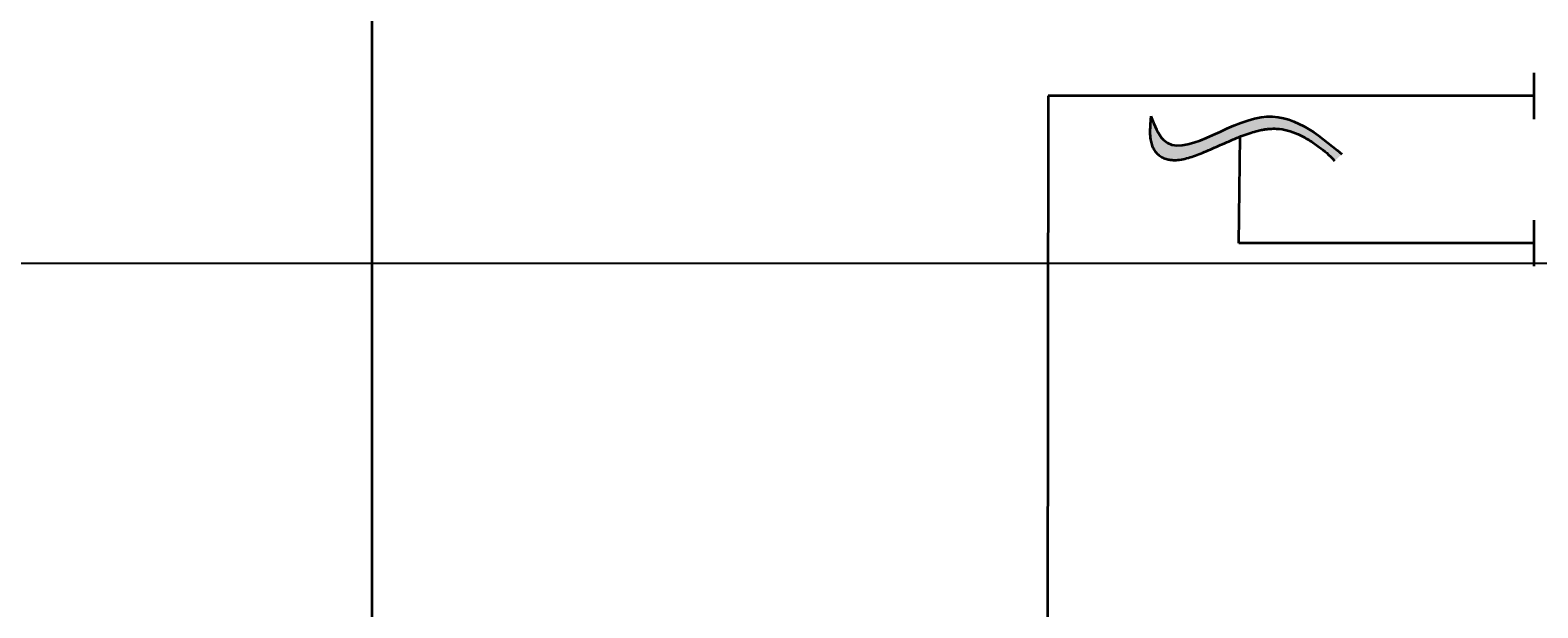
# Model space of a CAD drawing. Units: millimetres. Extents: x 353872 to 441597, y 126154 to 187356.
# Tile 16 of 28: x 391248 to 399262, y 158230 to 161299. Entities that reach past the tile are written whole.
import ezdxf

# ---------------------------------------------------------------- set-up
doc = ezdxf.new("R2010")
doc.units = ezdxf.units.MM
for name, color, linetype, lineweight in [('A-ANNO-DIMS', 2, 'Continuous', 18), ('P-PIPE', 3, 'Continuous', 35), ('P-SYMB-PATT', 8, 'Continuous', 13)]:
    doc.layers.add(name, color=color, linetype=linetype, lineweight=lineweight)
doc.styles.get("Standard").update_dxf_attribs({"font": 'arial.ttf'})
doc.dimstyles.get("Standard").update_dxf_attribs({"dimtxt": 0.18, "dimasz": 0.18, "dimexe": 0.18, "dimexo": 0.0625, "dimgap": 0.09, "dimtad": 0, "dimtih": 1, "dimtoh": 1, "dimdec": 4, "dimzin": 0, "dimdsep": 46, "dimtxsty": 'Standard', "dimcen": 0.09, "dimadec": 0, "dimazin": 0, "dimtfac": 1, "dimtdec": 4, "dimtofl": 0, "dimtmove": 0, "dimatfit": 3, "dimfxl": 1, "dimtolj": 1, "dimtzin": 0, "dimarcsym": 0})

# ---------------------------------------------------------------- blocks, each defined once
blk = doc.blocks.new('*D34')
at = {"layer": 'A-ANNO-DIMS', "color": 0, "lineweight": -2, "transparency": 16777216}
for p, q in [((399457.1, 167930), (356736.4, 167930)), ((356736.5, 167929.8), (356736.5, 163994.3)), ((356736.5, 160058.4), (356736.5, 163993.9)), ((399457.1, 160058.2), (356736.4, 160058.2))]:
    blk.add_line(p, q, dxfattribs=at)
at = {"layer": 'A-ANNO-DIMS', "color": 0, "transparency": 16777216}
for points in [[(356736.5, 167929.8), (356736.6, 167929.8), (356736.5, 167930)], [(356736.5, 160058.4), (356736.6, 160058.4), (356736.5, 160058.2)]]:
    blk.add_solid(points, dxfattribs=at)
at = {"layer": 'Defpoints', "color": 0, "transparency": 16777216}
for p in [(399457.2, 167930), (356736.5, 160058.2), (399457.2, 160058.2)]:
    blk.add_point(p, dxfattribs=at)
at = {"layer": 'A-ANNO-DIMS', "color": 0, "transparency": 16777216, "insert": (356736.5, 163994.1), "char_height": 0.18, "attachment_point": 5}
blk.add_mtext('\\A1;7872', dxfattribs=at)

msp = doc.modelspace()

# ---------------------------------------------------------------- hatches: boundary and pattern name
at = {"layer": 'P-SYMB-PATT'}
h = msp.add_hatch(color=256, dxfattribs=at)
h.dxf.hatch_style = 1
edge = h.paths.add_edge_path()
edge.add_spline(control_points=[(397205.05, 160842.23), (397204.61, 160837.28), (397204.16, 160832.26), (397202.84, 160817.1), (397202.01, 160806.84), (397200.63, 160785.35), (397200.12, 160774.12), (397199.95, 160751.62), (397200.28, 160740.37), (397202.07, 160722.7), (397202.95, 160716.44), (397205.13, 160705.42), (397206.25, 160700.71), (397209.06, 160691.15), (397210.73, 160686.4), (397215.91, 160673.98), (397219.95, 160666.4), (397229.78, 160652.11), (397235.58, 160645.42), (397248.52, 160633.66), (397255.64, 160628.59), (397270.38, 160620.36), (397277.98, 160617.19), (397293.04, 160612.45), (397300.51, 160610.88), (397315.1, 160608.89), (397322.23, 160608.47), (397342.23, 160608.42), (397354.76, 160609.77), (397379.55, 160614.04), (397391.81, 160616.99), (397416.54, 160624.05), (397428.98, 160628.15), (397454.23, 160637.22), (397467.03, 160642.19), (397507.59, 160658.66), (397536.01, 160671.23), (397593.65, 160696.76), (397622.85, 160709.71), (397680.46, 160733.58), (397708.87, 160744.49), (397748.65, 160757.34), (397761.14, 160760.99), (397781.84, 160766.23), (397790.28, 160768.11), (397805.08, 160770.91), (397811.57, 160771.94), (397824.38, 160773.59), (397830.66, 160774.21), (397849.19, 160775.48), (397861.12, 160775.55), (397893.15, 160773.86), (397912.63, 160770.68), (397950.84, 160760.7), (397969.58, 160753.87), (398006.91, 160736.94), (398025.48, 160726.84), (398062.71, 160703.97), (398081.36, 160691.2), (398126.14, 160658.54), (398152.38, 160637.8), (398181.22, 160603.69)], knot_values=[0, 0, 0, 0, 1.456577, 1.456577, 4.3697309, 4.3697309, 7.5343006, 7.5343006, 10.6988703, 10.6988703, 12.406712, 12.406712, 13.6390126, 13.6390126, 14.8713131, 14.8713131, 16.9006125, 16.9006125, 18.9299119, 18.9299119, 20.9592113, 20.9592113, 22.9885107, 22.9885107, 25.01781, 25.01781, 27.0471094, 27.0471094, 30.8253225, 30.8253225, 34.6035357, 34.6035357, 38.3817488, 38.3817488, 42.1599619, 42.1599619, 50.1898356, 50.1898356, 58.2197092, 58.2197092, 66.2495828, 66.2495828, 70.07412, 70.07412, 72.8401263, 72.8401263, 75.120346, 75.120346, 77.4005658, 77.4005658, 81.9610053, 81.9610053, 89.9551657, 89.9551657, 97.9493262, 97.9493262, 105.9434867, 105.9434867, 113.9376472, 113.9376472, 125.0020106, 125.0020106, 125.0020106, 125.0020106], degree=3, periodic=0)
edge.add_line((398181.22, 160603.69), (398220.74, 160639.63))
edge.add_spline(control_points=[(398220.74, 160639.63), (398088.6, 160749.8), (397930.06, 160881.99), (397724.17, 160821.47), (397689.5, 160808.66)], knot_values=[65.2965705, 65.2965705, 65.2965705, 65.2965705, 118.2135452, 128.7852065, 128.7852065, 128.7852065, 128.7852065], degree=3, periodic=0)
edge.add_spline(control_points=[(397689.5, 160808.66), (397527.98, 160749), (397302.36, 160591.22), (397224.26, 160792.68), (397205.05, 160842.23)], knot_values=[0, 0, 0, 0, 49.2381661, 65.2965705, 65.2965705, 65.2965705, 65.2965705], degree=3, periodic=0)

# ---------------------------------------------------------------- linework, layer by layer
at = {"layer": 'P-PIPE'}
for p, q in [((399242.2, 160826.46), (399242.2, 161071.22)), ((396659.16, 160948.84), (396648.15, 149319.73)), ((399242.2, 160948.84), (396659.16, 160948.84)), ((397671.76, 160166.82), (397680.5, 160733.28)), ((399242.2, 160044.44), (399242.2, 160289.2)), ((399242.2, 160166.82), (397671.76, 160166.82))]:
    msp.add_line(p, q, dxfattribs=at)
msp.add_lwpolyline([(393066.71, 149319.73), (393066.71, 175399.89), (426420.76, 175399.89)], dxfattribs=at)
for points, knots in [([(397205.05, 160842.23), (397204.61, 160837.28), (397204.16, 160832.26), (397202.84, 160817.1), (397202.01, 160806.84), (397200.63, 160785.35), (397200.12, 160774.12), (397199.95, 160751.62), (397200.28, 160740.37), (397202.07, 160722.7), (397202.95, 160716.44), (397205.13, 160705.42), (397206.25, 160700.71), (397209.06, 160691.15), (397210.73, 160686.4), (397215.91, 160673.98), (397219.95, 160666.4), (397229.78, 160652.11), (397235.58, 160645.42), (397248.52, 160633.66), (397255.64, 160628.59), (397270.38, 160620.36), (397277.98, 160617.19), (397293.04, 160612.45), (397300.51, 160610.88), (397315.1, 160608.89), (397322.23, 160608.47), (397342.23, 160608.42), (397354.76, 160609.77), (397379.55, 160614.04), (397391.81, 160616.99), (397416.54, 160624.05), (397428.98, 160628.15), (397454.23, 160637.22), (397467.03, 160642.19), (397507.59, 160658.66), (397536.01, 160671.23), (397593.65, 160696.76), (397622.85, 160709.71), (397680.46, 160733.58), (397708.87, 160744.49), (397748.65, 160757.34), (397761.14, 160760.99), (397781.84, 160766.23), (397790.28, 160768.11), (397805.08, 160770.91), (397811.57, 160771.94), (397824.38, 160773.59), (397830.66, 160774.21), (397849.19, 160775.48), (397861.12, 160775.55), (397893.15, 160773.86), (397912.63, 160770.68), (397950.84, 160760.7), (397969.58, 160753.87), (398006.91, 160736.94), (398025.48, 160726.84), (398062.71, 160703.97), (398081.36, 160691.2), (398126.14, 160658.54), (398152.38, 160637.8), (398181.22, 160603.69)], [0, 0, 0, 0, 1.456577, 1.456577, 4.3697309, 4.3697309, 7.5343006, 7.5343006, 10.6988703, 10.6988703, 12.406712, 12.406712, 13.6390126, 13.6390126, 14.8713131, 14.8713131, 16.9006125, 16.9006125, 18.9299119, 18.9299119, 20.9592113, 20.9592113, 22.9885107, 22.9885107, 25.01781, 25.01781, 27.0471094, 27.0471094, 30.8253225, 30.8253225, 34.6035357, 34.6035357, 38.3817488, 38.3817488, 42.1599619, 42.1599619, 50.1898356, 50.1898356, 58.2197092, 58.2197092, 66.2495828, 66.2495828, 70.07412, 70.07412, 72.8401263, 72.8401263, 75.120346, 75.120346, 77.4005658, 77.4005658, 81.9610053, 81.9610053, 89.9551657, 89.9551657, 97.9493262, 97.9493262, 105.9434867, 105.9434867, 113.9376472, 113.9376472, 125.0020106, 125.0020106, 125.0020106, 125.0020106]), ([(397205.05, 160842.23), (397224.26, 160792.68), (397315, 160558.6), (397807.1, 160984.5), (398088.6, 160749.8), (398220.74, 160639.63)], [0, 0, 0, 0, 143.2990836, 677.0191991, 1149.2301239, 1149.2301239, 1149.2301239, 1149.2301239])]:
    msp.add_open_spline(points, degree=3, knots=knots, dxfattribs=at)

# ---------------------------------------------------------------- dimensions: what is measured, and where the dimension line sits
at = {"layer": 'A-ANNO-DIMS'}
dim = msp.add_linear_dim(base=(356736.55, 160058.19), p1=(399457.15, 167929.97), p2=(399457.15, 160058.19), angle=90, dimstyle='Standard', override={"dimdec": 0, "dimlfac": 1, "dimrnd": 0, "dimzin": 0, "dimdsep": 46, "dimlunit": 2}, dxfattribs=at)
dim.commit()
dim.dimension.update_dxf_attribs({"geometry": '*D34', "text_midpoint": (356736.55, 163994.08)})

doc.saveas('drawing.dxf')
